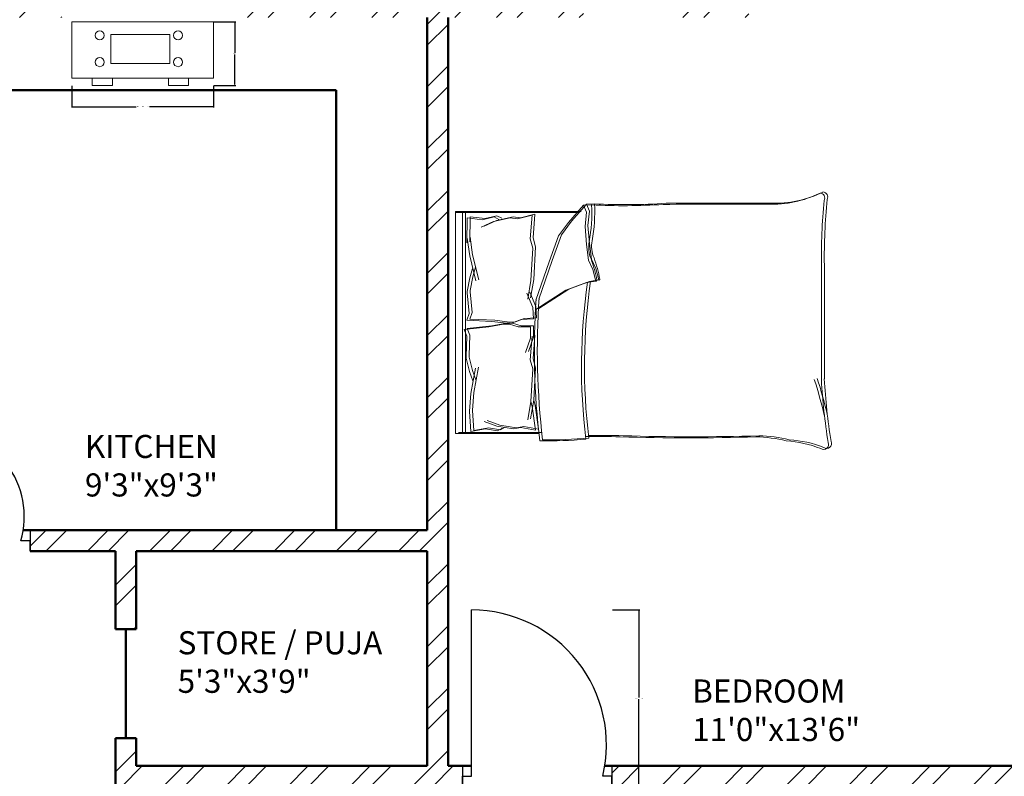
# Model space of a CAD drawing. Units: inches. Extents: x 963 to 2075, y 289 to 2657.
# Tile 96 of 98: x 1672 to 1885, y 2325 to 2489. Entities that reach past the tile are written whole.
import ezdxf

# ---------------------------------------------------------------- set-up
doc = ezdxf.new("R2010")
doc.units = ezdxf.units.IN
for name, color, linetype, lineweight in [('A-ANNO-DIMS', 2, 'Continuous', 18), ('A-AREA-IDEN', 7, 'Continuous', 18), ('A-DOOR', 4, 'Continuous', 25), ('A-FLOR-FIXT', 9, 'Continuous', 18), ('A-FURN', 8, 'Continuous', 18), ('A-WALL', 7, 'Continuous', 50), ('A-WALL-PATT', 8, 'Continuous', 13)]:
    doc.layers.add(name, color=color, linetype=linetype, lineweight=lineweight)
doc.styles.get("Standard").update_dxf_attribs({"font": 'arial.ttf'})
doc.dimstyles.get("Standard").update_dxf_attribs({"dimtxt": 0.18, "dimasz": 0.18, "dimexe": 0.18, "dimexo": 0.0625, "dimgap": 0.09, "dimtad": 0, "dimtih": 1, "dimtoh": 1, "dimdec": 4, "dimzin": 0, "dimdsep": 46, "dimtxsty": 'Standard', "dimcen": 0.09, "dimadec": 0, "dimazin": 0, "dimtfac": 1, "dimtdec": 4, "dimtofl": 0, "dimtmove": 0, "dimatfit": 3, "dimfxl": 1, "dimtolj": 1, "dimtzin": 0, "dimarcsym": 0})

# ---------------------------------------------------------------- blocks, each defined once
blk = doc.blocks.new('BED-DOUBLE')
for p, q in [((1236.12, 2450.52), (1254.23, 2450.52)), ((1236.12, 2450.52), (1254.23, 2450.52)), ((1236.76, 2450.75), (1254.87, 2450.75)), ((1236.76, 2450.75), (1254.87, 2450.75)), ((1238.25, 2444.94), (1237.53, 2450.04)), ((1237.53, 2450.04), (1240.71, 2449.46)), ((1238.25, 2444.94), (1237.53, 2450.04)), ((1237.53, 2450.04), (1240.71, 2449.46)), ((1245.77, 2450.18), (1244.76, 2449.61)), ((1245.77, 2450.18), (1244.76, 2449.61)), ((1248.37, 2449.75), (1245.77, 2450.18)), ((1248.37, 2449.75), (1245.77, 2450.18)), ((1250.92, 2450.1), (1247.74, 2449.52)), ((1250.92, 2450.1), (1247.74, 2449.52)), ((1251.56, 2450.33), (1248.37, 2449.75)), ((1251.56, 2450.33), (1248.37, 2449.75)), ((1250.89, 2450.1), (1251.22, 2445.82)), ((1250.89, 2450.1), (1251.22, 2445.82)), ((1251.53, 2450.32), (1251.86, 2446.04)), ((1251.53, 2450.32), (1251.86, 2446.04)), ((1252.7, 2450.52), (1252.7, 2402.73)), ((1252.7, 2450.52), (1252.7, 2402.73)), ((1253.34, 2450.75), (1253.34, 2402.96)), ((1253.34, 2450.75), (1253.34, 2402.96)), ((1254.87, 2450.75), (1254.87, 2402.73)), ((1237.61, 2444.71), (1236.89, 2449.81)), ((1236.89, 2449.81), (1240.07, 2449.23)), ((1237.61, 2444.71), (1236.89, 2449.81)), ((1236.89, 2449.81), (1240.07, 2449.23)), ((1240.07, 2449.23), (1241.66, 2449.52)), ((1240.07, 2449.23), (1241.66, 2449.52)), ((1240.71, 2449.46), (1242.3, 2449.75)), ((1240.71, 2449.46), (1242.3, 2449.75)), ((1241.66, 2449.52), (1245.28, 2448.94)), ((1241.66, 2449.52), (1245.28, 2448.94)), ((1242.3, 2449.75), (1245.92, 2449.17)), ((1242.3, 2449.75), (1245.92, 2449.17)), ((1245.13, 2449.96), (1244.12, 2449.38)), ((1245.13, 2449.96), (1244.12, 2449.38)), ((1247.74, 2449.52), (1245.13, 2449.96)), ((1247.74, 2449.52), (1245.13, 2449.96)), ((1245.28, 2448.94), (1248.02, 2447.93)), ((1245.28, 2448.94), (1248.02, 2447.93)), ((1245.92, 2449.17), (1248.66, 2448.16)), ((1245.92, 2449.17), (1248.66, 2448.16)), ((1238.6, 2447.61), (1237.94, 2443.58)), ((1238.6, 2447.61), (1237.94, 2443.58)), ((1239.24, 2447.84), (1238.58, 2443.81)), ((1239.24, 2447.84), (1238.58, 2443.81)), ((1251.22, 2445.82), (1251.21, 2445.71)), ((1251.22, 2445.82), (1251.21, 2445.71)), ((1251.84, 2445.94), (1251.56, 2442.11)), ((1251.84, 2445.94), (1251.56, 2442.11)), ((1251.86, 2446.04), (1251.84, 2445.94)), ((1251.86, 2446.04), (1251.84, 2445.94)), ((1237.94, 2443.58), (1237.61, 2444.71)), ((1237.94, 2443.58), (1237.61, 2444.71)), ((1238.58, 2443.81), (1238.15, 2436.8)), ((1238.58, 2443.81), (1238.15, 2436.8)), ((1238.58, 2443.81), (1238.25, 2444.94)), ((1238.58, 2443.81), (1238.25, 2444.94)), ((1251.21, 2445.71), (1250.92, 2441.89)), ((1251.21, 2445.71), (1250.92, 2441.89)), ((1237.94, 2443.58), (1237.51, 2436.57)), ((1237.94, 2443.58), (1237.51, 2436.57)), ((1250.92, 2441.89), (1249.9, 2436.39)), ((1250.92, 2441.89), (1249.9, 2436.39)), ((1251.56, 2442.11), (1250.54, 2436.62)), ((1251.56, 2442.11), (1250.54, 2436.62)), ((1251.12, 2439.37), (1251.84, 2437.34)), ((1251.12, 2439.37), (1251.84, 2437.34)), ((1174.99, 2438.93), (1174.99, 2414.32)), ((1174.99, 2438.93), (1174.99, 2414.32)), ((1175.63, 2439.16), (1175.63, 2414.55)), ((1175.63, 2439.16), (1175.63, 2414.55)), ((1250.48, 2439.14), (1251.21, 2437.12)), ((1250.48, 2439.14), (1251.21, 2437.12)), ((1251.84, 2437.34), (1252.57, 2434.45)), ((1251.84, 2437.34), (1252.57, 2434.45)), ((1237.51, 2436.57), (1238.06, 2434.61)), ((1237.51, 2436.57), (1238.06, 2434.61)), ((1238.15, 2436.8), (1238.7, 2434.84)), ((1238.15, 2436.8), (1238.7, 2434.84)), ((1251.21, 2437.12), (1251.93, 2434.22)), ((1251.21, 2437.12), (1251.93, 2434.23)), ((1238.06, 2434.61), (1237.66, 2429.48)), ((1238.06, 2434.61), (1237.66, 2429.48)), ((1237.97, 2429.89), (1239.06, 2433.04)), ((1237.97, 2429.89), (1239.06, 2433.04)), ((1238.7, 2434.84), (1238.3, 2429.71)), ((1238.7, 2434.84), (1238.3, 2429.71)), ((1238.61, 2430.12), (1239.7, 2433.26)), ((1238.61, 2430.12), (1239.7, 2433.26)), ((1251.93, 2433.9), (1251.78, 2429.46)), ((1251.93, 2433.9), (1251.78, 2429.46)), ((1251.93, 2434.23), (1251.93, 2433.9)), ((1251.93, 2434.22), (1251.93, 2433.9)), ((1252.57, 2434.13), (1252.42, 2429.69)), ((1252.57, 2434.13), (1252.42, 2429.69)), ((1252.57, 2434.45), (1252.57, 2434.13)), ((1252.57, 2434.45), (1252.57, 2434.13)), ((1237.97, 2427.43), (1237.97, 2429.89)), ((1237.97, 2427.43), (1237.97, 2429.89)), ((1238.61, 2427.66), (1238.61, 2430.12)), ((1238.61, 2427.66), (1238.61, 2430.12)), ((1251.78, 2429.46), (1252.36, 2428.01)), ((1251.78, 2429.46), (1252.36, 2428.01)), ((1252.42, 2429.69), (1253, 2428.24)), ((1252.42, 2429.69), (1253, 2428.24)), ((1240.65, 2427.43), (1237.97, 2427.43)), ((1240.65, 2427.43), (1237.97, 2427.43)), ((1241.29, 2427.66), (1238.61, 2427.66)), ((1241.29, 2427.66), (1238.61, 2427.66)), ((1242.53, 2426.86), (1240.65, 2427.43)), ((1242.53, 2426.86), (1240.65, 2427.43)), ((1242.49, 2426.79), (1240.66, 2426.09)), ((1242.49, 2426.79), (1240.66, 2426.09)), ((1243.17, 2427.08), (1241.29, 2427.66)), ((1243.17, 2427.08), (1241.29, 2427.66)), ((1243.15, 2426.64), (1241.86, 2426.56)), ((1243.15, 2426.64), (1241.86, 2426.56)), ((1243.79, 2426.87), (1242.49, 2426.79)), ((1243.79, 2426.87), (1242.49, 2426.79)), ((1243.83, 2426.86), (1242.53, 2426.86)), ((1243.83, 2426.86), (1242.53, 2426.86)), ((1246.37, 2426.26), (1243.15, 2426.64)), ((1246.37, 2426.26), (1243.15, 2426.64)), ((1244.47, 2427.08), (1243.17, 2427.08)), ((1244.47, 2427.08), (1243.17, 2427.08)), ((1247, 2426.49), (1243.79, 2426.87)), ((1247, 2426.49), (1243.79, 2426.87)), ((1247.01, 2427.43), (1243.83, 2426.86)), ((1247.01, 2427.43), (1243.83, 2426.86)), ((1247.65, 2427.66), (1244.47, 2427.08)), ((1247.65, 2427.66), (1244.47, 2427.08)), ((1252.36, 2428.01), (1247.01, 2427.43)), ((1252.36, 2428.01), (1247.01, 2427.43)), ((1253, 2428.24), (1247.65, 2427.66)), ((1253, 2428.24), (1247.65, 2427.66)), ((1240.02, 2425.86), (1237.34, 2425.7)), ((1240.02, 2425.86), (1237.34, 2425.7)), ((1237.34, 2425.7), (1237.49, 2423.24)), ((1237.34, 2425.7), (1237.49, 2423.24)), ((1240.66, 2426.09), (1237.98, 2425.93)), ((1240.66, 2426.09), (1237.98, 2425.93)), ((1237.98, 2425.93), (1238.13, 2423.47)), ((1237.98, 2425.93), (1238.13, 2423.47)), ((1241.86, 2426.56), (1240.02, 2425.86)), ((1241.86, 2426.56), (1240.02, 2425.86)), ((1251.74, 2426.02), (1246.37, 2426.26)), ((1251.74, 2426.02), (1246.37, 2426.26)), ((1252.38, 2426.25), (1247, 2426.49)), ((1252.38, 2426.25), (1247, 2426.49)), ((1251.25, 2424.54), (1251.74, 2426.02)), ((1251.25, 2424.54), (1251.74, 2426.02)), ((1251.68, 2420.11), (1251.25, 2424.54)), ((1251.68, 2420.11), (1251.25, 2424.54)), ((1251.89, 2424.77), (1252.38, 2426.25)), ((1251.89, 2424.77), (1252.38, 2426.25)), ((1252.31, 2420.34), (1251.89, 2424.77)), ((1252.31, 2420.34), (1251.89, 2424.77)), ((1236.85, 2423.74), (1230.36, 2419.55)), ((1236.85, 2423.74), (1230.36, 2419.55)), ((1237.49, 2423.96), (1231, 2419.77)), ((1237.49, 2423.96), (1231, 2419.77)), ((1237.49, 2423.24), (1238.78, 2420.17)), ((1237.49, 2423.24), (1238.78, 2420.17)), ((1238.13, 2423.47), (1239.42, 2420.4)), ((1238.13, 2423.47), (1239.42, 2420.4)), ((1233.92, 2413.35), (1236.85, 2421.69)), ((1233.92, 2413.35), (1236.85, 2421.69)), ((1234.56, 2413.58), (1237.49, 2421.92)), ((1234.56, 2413.58), (1237.49, 2421.92)), ((1238.6, 2421.43), (1237.94, 2417.4)), ((1238.6, 2421.43), (1237.94, 2417.4)), ((1239.24, 2421.66), (1238.58, 2417.63)), ((1239.24, 2421.66), (1238.58, 2417.63)), ((1252.33, 2420.02), (1252.31, 2420.34)), ((1252.33, 2420.02), (1252.31, 2420.34)), ((1226.51, 2418.07), (1224.49, 2417.76)), ((1226.51, 2418.07), (1224.49, 2417.76)), ((1230.36, 2419.55), (1225.87, 2417.84)), ((1230.36, 2419.55), (1225.87, 2417.84)), ((1231, 2419.77), (1226.51, 2418.07)), ((1231, 2419.77), (1226.51, 2418.07)), ((1251.15, 2416.86), (1251.7, 2419.79)), ((1251.15, 2416.86), (1251.7, 2419.79)), ((1251.7, 2419.79), (1251.68, 2420.11)), ((1251.7, 2419.79), (1251.68, 2420.11)), ((1251.79, 2417.09), (1252.33, 2420.02)), ((1251.79, 2417.09), (1252.33, 2420.02)), ((1225.87, 2417.84), (1223.86, 2417.53)), ((1225.87, 2417.84), (1223.86, 2417.53)), ((1223.86, 2417.53), (1224.47, 2415.05)), ((1223.86, 2417.53), (1224.47, 2415.05)), ((1224.49, 2417.76), (1225.11, 2415.28)), ((1224.49, 2417.76), (1225.11, 2415.28)), ((1237.94, 2417.4), (1237.51, 2410.39)), ((1237.94, 2417.4), (1237.51, 2410.39)), ((1238.58, 2417.63), (1238.15, 2410.62)), ((1238.58, 2417.63), (1238.15, 2410.62)), ((1251.16, 2412.08), (1249.81, 2417.5)), ((1251.16, 2412.08), (1249.81, 2417.5)), ((1251.8, 2412.31), (1250.45, 2417.73)), ((1251.8, 2412.31), (1250.45, 2417.73)), ((1250.56, 2414.79), (1251.15, 2416.86)), ((1250.56, 2414.79), (1251.15, 2416.86)), ((1251.2, 2415.02), (1251.79, 2417.09)), ((1251.2, 2415.02), (1251.79, 2417.09)), ((1224.47, 2415.05), (1225.4, 2413.04)), ((1224.47, 2415.05), (1225.4, 2413.04)), ((1225.11, 2415.28), (1226.04, 2413.27)), ((1225.11, 2415.28), (1226.04, 2413.27)), ((1225.4, 2413.04), (1225.87, 2409.63)), ((1225.4, 2413.04), (1225.87, 2409.63)), ((1226.04, 2413.27), (1226.51, 2409.86)), ((1226.04, 2413.27), (1226.51, 2409.86)), ((1231.9, 2407.77), (1233.92, 2413.35)), ((1231.9, 2407.78), (1233.92, 2413.35)), ((1232.54, 2408), (1234.56, 2413.58)), ((1232.54, 2408), (1234.56, 2413.58)), ((1251.69, 2408.28), (1251.16, 2412.08)), ((1251.69, 2408.28), (1251.16, 2412.08)), ((1252.33, 2408.51), (1251.8, 2412.31)), ((1252.33, 2408.51), (1251.8, 2412.31)), ((1225.87, 2409.63), (1226.18, 2405.76)), ((1225.87, 2409.63), (1226.18, 2405.76)), ((1226.51, 2409.86), (1226.82, 2405.99)), ((1226.51, 2409.86), (1226.82, 2405.99)), ((1237.51, 2410.39), (1238.06, 2408.43)), ((1237.51, 2410.39), (1238.06, 2408.43)), ((1238.15, 2410.62), (1238.7, 2408.66)), ((1238.15, 2410.62), (1238.7, 2408.66)), ((1252.31, 2404.11), (1252.41, 2409.51)), ((1252.31, 2404.11), (1252.41, 2409.51)), ((1252.41, 2409.51), (1252.33, 2408.51)), ((1252.41, 2409.51), (1252.33, 2408.51)), ((1229.74, 2404.83), (1231.9, 2407.78)), ((1229.74, 2404.83), (1231.9, 2407.77)), ((1230.38, 2405.06), (1232.54, 2408)), ((1230.38, 2405.06), (1232.54, 2408)), ((1238.06, 2408.43), (1237.66, 2403.3)), ((1238.06, 2408.43), (1237.66, 2403.3)), ((1238.7, 2408.66), (1238.3, 2403.52)), ((1238.7, 2408.66), (1238.3, 2403.52)), ((1251.68, 2403.88), (1251.77, 2409.29)), ((1251.68, 2403.88), (1251.77, 2409.28)), ((1251.77, 2409.29), (1251.69, 2408.28)), ((1251.77, 2409.28), (1251.69, 2408.28)), ((1226.18, 2405.76), (1225.87, 2402.66)), ((1226.18, 2405.76), (1225.87, 2402.66)), ((1226.82, 2405.99), (1226.51, 2402.89)), ((1226.82, 2405.99), (1226.51, 2402.89)), ((1245.98, 2404.69), (1248.65, 2405.87)), ((1245.98, 2404.69), (1248.65, 2405.87)), ((1246.61, 2404.91), (1249.29, 2406.1)), ((1246.61, 2404.91), (1249.29, 2406.09)), ((1226.49, 2401.13), (1229.74, 2404.83)), ((1226.49, 2401.13), (1229.74, 2404.83)), ((1227.13, 2401.36), (1230.38, 2405.06)), ((1227.13, 2401.36), (1230.38, 2405.06)), ((1237.66, 2403.3), (1240.8, 2404.07)), ((1237.66, 2403.3), (1240.8, 2404.07)), ((1238.3, 2403.52), (1241.44, 2404.3)), ((1238.3, 2403.52), (1241.44, 2404.3)), ((1240.8, 2404.07), (1242.4, 2403.88)), ((1240.8, 2404.07), (1242.4, 2403.88)), ((1241.44, 2404.3), (1243.04, 2404.11)), ((1241.44, 2404.3), (1243.04, 2404.11)), ((1242.4, 2403.88), (1245.98, 2404.69)), ((1242.4, 2403.88), (1245.98, 2404.69)), ((1243.04, 2404.11), (1246.61, 2404.91)), ((1243.04, 2404.11), (1246.61, 2404.91)), ((1245.89, 2403.67), (1244.85, 2404.18)), ((1245.89, 2403.67), (1244.85, 2404.18)), ((1246.53, 2403.89), (1245.49, 2404.41)), ((1246.53, 2403.89), (1245.49, 2404.41)), ((1248.46, 2404.26), (1245.89, 2403.67)), ((1248.46, 2404.26), (1245.89, 2403.67)), ((1249.1, 2404.49), (1246.53, 2403.89)), ((1249.1, 2404.49), (1246.53, 2403.89)), ((1251.68, 2403.88), (1248.46, 2404.26)), ((1251.68, 2403.88), (1248.46, 2404.26)), ((1252.31, 2404.11), (1249.1, 2404.49)), ((1252.31, 2404.11), (1249.1, 2404.49)), ((1224.74, 2401.05), (1226.49, 2401.13, 3.87)), ((1224.74, 2401.05), (1226.49, 2401.13, 3.87)), ((1225.38, 2401.28), (1227.13, 2401.36, 3.87)), ((1225.38, 2401.28), (1227.13, 2401.36, 3.87)), ((1225.87, 2402.66), (1226.49, 2401.13)), ((1225.87, 2402.66), (1226.49, 2401.13)), ((1226.51, 2402.89), (1227.13, 2401.36)), ((1226.51, 2402.89), (1227.13, 2401.36)), ((1254.23, 2402.73), (1227.62, 2402.73)), ((1254.23, 2402.73), (1227.62, 2402.73)), ((1254.87, 2402.96), (1228.26, 2402.96)), ((1254.87, 2402.96), (1228.26, 2402.96)), ((1254.87, 2402.73), (1254.23, 2402.73))]:
    blk.add_line(p, q)
for centre, radius, start, end in [((1174.51, 2452.91), 1.09, 56.1736, 203.4781), ((1174.51, 2452.91), 1.09, 56.1736, 203.4781), ((1053.4, 2432.57), 121.76, 2.9958, 9.4091), ((1053.4, 2432.57), 121.76, 2.9958, 9.4091), ((1175.15, 2453.14), 1.09, 56.1736, 203.4781), ((1175.15, 2453.14), 1.09, 56.1736, 203.4781), ((1054.03, 2432.8), 121.76, 2.9958, 9.4091), ((1054.03, 2432.8), 121.76, 2.9958, 9.4091), ((1183.96, 2475.65), 23.56, 247.9751, 266.652), ((1183.96, 2475.65), 23.56, 247.9751, 266.652), ((1184.6, 2475.88), 23.56, 247.9751, 266.652), ((1184.6, 2475.88), 23.56, 247.9751, 266.652), ((1190.36, 2481.12), 29.63, 256.0648, 268.9113), ((1190.36, 2481.12), 29.63, 256.0648, 268.9113), ((1234.78, 2369.06), 83.31, 88.7218, 95.604), ((1234.78, 2369.06), 83.31, 88.7218, 95.604), ((1072.82, 2432.86), 164.97, 356.0865, 6.7821), ((1072.82, 2432.86), 164.97, 356.0865, 6.7821), ((1189.72, 2480.89), 29.63, 256.0648, 268.9113), ((1189.72, 2480.89), 29.63, 256.0648, 268.9113), ((1203.62, 1969.17), 482.31, 88.2277, 91.7185), ((1203.62, 1969.17), 482.31, 88.2277, 91.7185), ((1204.26, 1969.4), 482.31, 88.2277, 91.7185), ((1204.26, 1969.4), 482.31, 88.2277, 91.7185), ((1223.06, 2621.3), 170.11, 268.4762, 271.0082), ((1223.06, 2621.3), 170.11, 268.4762, 271.0082), ((1223.7, 2621.53), 170.11, 268.4762, 271.0082), ((1223.7, 2621.53), 170.11, 268.4762, 271.0082), ((1097.92, 2436.24), 129.02, 351.7845, 6.9006), ((1097.92, 2436.24), 129.02, 351.7845, 6.9006), ((1234.14, 2368.83), 83.31, 88.7218, 95.604), ((1234.14, 2368.83), 83.31, 88.7218, 95.604), ((1098.56, 2436.47), 129.02, 351.7845, 6.9006), ((1098.56, 2436.47), 129.02, 351.7845, 6.9006), ((1072.18, 2432.64), 164.97, 356.0865, 6.7821), ((1072.18, 2432.64), 164.97, 356.0865, 6.7821), ((1277.94, 2471.22), 106.46, 193.3832, 197.7053), ((1277.94, 2471.22), 106.46, 193.3832, 197.7053), ((1278.58, 2471.44), 106.46, 193.3832, 197.7053), ((1278.58, 2471.44), 106.46, 193.3832, 197.7053), ((1223.79, 2417.36), 0.185, 70.2464, 181.1377), ((1223.79, 2417.36), 0.185, 70.2464, 181.1377), ((1252.75, 2422.84), 29.65, 190.6617, 199.8806), ((1252.75, 2422.84), 29.65, 190.6617, 199.8806), ((1224.43, 2417.59), 0.185, 70.2464, 181.1377), ((1224.43, 2417.59), 0.185, 70.2464, 181.1377), ((1253.39, 2423.07), 29.65, 190.6617, 199.8806), ((1253.39, 2423.07), 29.65, 190.6617, 199.8806), ((1041.96, 2412.84), 133.04, 354.4998, 0.6351), ((1041.96, 2412.84), 133.04, 354.4998, 0.6351), ((1042.6, 2413.07), 133.04, 354.4998, 0.6351), ((1042.6, 2413.07), 133.04, 354.4998, 0.6351), ((1219.17, 2410.25), 6.22, 348.6608, 23.7384), ((1219.17, 2410.25), 6.22, 348.6608, 23.7384), ((1219.81, 2410.48), 6.22, 348.6608, 23.7384), ((1219.81, 2410.48), 6.22, 348.6608, 23.7384), ((1260.89, 2402.67), 36.18, 169.8763, 182.5657), ((1260.89, 2402.67), 36.18, 169.8763, 182.5657), ((1261.53, 2402.9), 36.18, 169.8763, 182.5657), ((1261.53, 2402.9), 36.18, 169.8763, 182.5657), ((1186.21, 2378.07), 23.07, 87.4714, 116.4681), ((1186.21, 2378.07), 23.07, 87.4714, 116.4681), ((1187.05, 6962.97), 4561.86, 270.00217, 270.28689), ((1187.05, 6962.97), 4561.86, 270.00217, 270.28689), ((1217.92, 2271.73), 129.5, 86.9791, 93.8365), ((1217.92, 2271.73), 129.5, 86.9791, 93.8365), ((1218.56, 2271.96), 129.5, 86.9791, 93.8365), ((1218.56, 2271.96), 129.5, 86.9791, 93.8365), ((1175.36, 2399.58), 1.1, 152.6588, 266.02), ((1175.36, 2399.58), 1.1, 152.6588, 266.02), ((1176, 2399.81), 1.1, 152.6588, 266.02), ((1176, 2399.81), 1.1, 152.6588, 266.02), ((1185.57, 2377.84), 23.07, 87.4714, 116.4681), ((1185.57, 2377.84), 23.07, 87.4714, 116.4681), ((1186.41, 6962.74), 4561.86, 270.00217, 270.28689), ((1186.41, 6962.74), 4561.86, 270.00217, 270.28689)]:
    blk.add_arc(centre, radius, start, end)
blk = doc.blocks.new('KITCHEN-SINK')
for points in [[(-0.1, 14), (30.59, 14), (30.59, 1.84), (-0.1, 1.84)], [(8.33, 11.28), (21.1, 11.28), (21.1, 5.02), (8.33, 5.02)], [(4.31, 1.84), (8.69, 1.84), (8.69, 0.24), (4.31, 0.24)], [(20.79, 1.84), (25.17, 1.84), (25.17, 0.24), (20.79, 0.24)]]:
    blk.add_lwpolyline(points, close=True)
for centre in [(5.94, 11.08), (22.9, 11.08), (5.94, 5.28), (22.9, 5.28)]:
    blk.add_circle(centre, 0.978)
blk = doc.blocks.new('DOOR-3')
for p, q in [((2, 2.25), (2, 38.25)), ((0, 4.5), (0, 0)), ((32.39, 4.5), (32.39, 0)), ((0, 0), (0, 2.25)), ((0, 2.25), (2, 2.25)), ((32.39, 2.25), (30.39, 2.25)), ((32.39, 0), (32.39, 2.25))]:
    blk.add_line(p, q)
blk.add_arc((2, 9.06), 29.19, 346.5105, 90)
blk = doc.blocks.new('*D20')
at = {"layer": 'A-ANNO-DIMS', "color": 0, "lineweight": -2, "transparency": 16777216}
for p, q in [((1683.48, 2474.56), (1683.48, 2469.84)), ((1714.16, 2474.56), (1714.16, 2469.84)), ((1683.66, 2470.02), (1697.38, 2470.02)), ((1713.98, 2470.02), (1700.26, 2470.02))]:
    blk.add_line(p, q, dxfattribs=at)
at = {"layer": 'A-ANNO-DIMS', "color": 0, "transparency": 16777216}
for points in [[(1683.66, 2470.05), (1683.66, 2469.99), (1683.48, 2470.02)], [(1713.98, 2470.05), (1713.98, 2469.99), (1714.16, 2470.02)]]:
    blk.add_solid(points, dxfattribs=at)
at = {"layer": 'Defpoints', "color": 0, "transparency": 16777216}
for p in [(1683.48, 2474.62), (1714.16, 2474.62), (1714.16, 2470.02)]:
    blk.add_point(p, dxfattribs=at)
at = {"layer": 'A-ANNO-DIMS', "color": 0, "transparency": 16777216, "insert": (1698.82, 2470.02), "char_height": 0.18, "attachment_point": 5}
blk.add_mtext('\\A1;KITCHEN SINK 31 TYP.', dxfattribs=at)
blk = doc.blocks.new('*D21')
at = {"layer": 'A-ANNO-DIMS', "color": 0, "lineweight": -2, "transparency": 16777216}
for p, q in [((1714.23, 2488.38), (1718.95, 2488.38)), ((1718.77, 2488.2), (1718.77, 2481.68)), ((1718.77, 2474.8), (1718.77, 2481.32)), ((1714.23, 2474.62), (1718.95, 2474.62))]:
    blk.add_line(p, q, dxfattribs=at)
at = {"layer": 'A-ANNO-DIMS', "color": 0, "transparency": 16777216}
for points in [[(1718.74, 2488.2), (1718.8, 2488.2), (1718.77, 2488.38)], [(1718.74, 2474.8), (1718.8, 2474.8), (1718.77, 2474.62)]]:
    blk.add_solid(points, dxfattribs=at)
at = {"layer": 'Defpoints', "color": 0, "transparency": 16777216}
for p in [(1714.16, 2488.38), (1718.77, 2488.38), (1714.16, 2474.62)]:
    blk.add_point(p, dxfattribs=at)
at = {"layer": 'A-ANNO-DIMS', "color": 0, "transparency": 16777216, "insert": (1718.77, 2481.5), "char_height": 0.18, "attachment_point": 5}
blk.add_mtext('\\A1;14 TYP.', dxfattribs=at)
blk = doc.blocks.new('*D34')
at = {"layer": 'A-ANNO-DIMS', "color": 0, "lineweight": -2, "transparency": 16777216}
for p, q in [((1800.57, 2361.07), (1806.43, 2361.07)), ((1806.25, 2360.89), (1806.25, 2342.13)), ((1806.25, 2323), (1806.25, 2341.76)), ((1800.57, 2322.82), (1806.43, 2322.82))]:
    blk.add_line(p, q, dxfattribs=at)
at = {"layer": 'A-ANNO-DIMS', "color": 0, "transparency": 16777216}
for points in [[(1806.22, 2360.89), (1806.28, 2360.89), (1806.25, 2361.07)], [(1806.22, 2323), (1806.28, 2323), (1806.25, 2322.82)]]:
    blk.add_solid(points, dxfattribs=at)
at = {"layer": 'Defpoints', "color": 0, "transparency": 16777216}
for p in [(1800.51, 2361.07), (1806.25, 2361.07), (1800.51, 2322.82)]:
    blk.add_point(p, dxfattribs=at)
at = {"layer": 'A-ANNO-DIMS', "color": 0, "transparency": 16777216, "insert": (1806.25, 2341.94), "char_height": 0.18, "attachment_point": 5}
blk.add_mtext('\\A1;DOOR D3 38 TYP.', dxfattribs=at)

msp = doc.modelspace()

# ---------------------------------------------------------------- hatches: boundary and pattern name
at = {"layer": 'A-WALL-PATT'}
h = msp.add_hatch(dxfattribs=at)
h.set_pattern_fill('ANSI32', color=256)
h.paths.add_polyline_path([(1296.92, 2558.32), (1203.92, 2558.32), (1203.92, 2493.82), (1191.53, 2493.82), (1191.53, 2489.32), (1211.06, 2489.32), (1211.06, 2492.02), (1211.06, 2493.82), (1208.42, 2493.82), (1208.42, 2553.82), (1292.42, 2553.82), (1292.42, 2538.86), (1296.92, 2538.86)])
h.paths.add_polyline_path([(1442.42, 2558.32), (1349.42, 2558.32), (1349.42, 2538.94), (1353.92, 2538.94), (1353.92, 2553.82), (1437.92, 2553.82), (1437.92, 2493.82), (1434.54, 2493.82), (1434.54, 2489.32), (1448.31, 2489.32), (1448.31, 2491.57), (1448.31, 2493.82), (1442.42, 2493.82)])
h.paths.add_polyline_path([(1415.55, 2491.57), (1415.55, 2493.82), (1340.94, 2493.82), (1340.94, 2489.32), (1371.92, 2489.32), (1371.92, 2378.32), (1367.6, 2378.32), (1367.6, 2373.82), (1371.92, 2373.82), (1371.92, 2355.19), (1376.42, 2355.19), (1376.42, 2489.32), (1415.55, 2489.32)])
h.paths.add_polyline_path([(1304.94, 2491.57), (1304.94, 2493.82), (1296.92, 2493.82), (1296.92, 2514.86), (1292.42, 2514.86), (1292.42, 2493.82), (1232.81, 2493.82), (1232.81, 2489.32), (1256.42, 2489.32), (1256.42, 2327.32), (1253.71, 2327.32), (1253.71, 2322.82), (1328.42, 2322.82), (1328.42, 2331.15), (1323.92, 2331.15), (1323.92, 2327.32), (1260.92, 2327.32), (1260.92, 2373.82), (1323.92, 2373.82), (1323.92, 2357.81), (1328.42, 2357.81), (1328.42, 2373.82), (1346.01, 2373.82), (1346.01, 2376.07), (1346.01, 2378.32), (1260.92, 2378.32), (1260.92, 2489.32), (1304.94, 2489.32)])
h.paths.add_polyline_path([(1226.65, 2327.32), (1124.42, 2327.32), (1124.42, 2347.45), (1119.92, 2347.45), (1119.92, 2322.82), (1163.42, 2322.82), (1163.42, 2305.43), (1165.67, 2305.43), (1167.92, 2305.43), (1167.92, 2322.82), (1226.65, 2322.82), (1226.65, 2325.07)])
h.paths.add_polyline_path([(1095.92, 2489.32), (1124.42, 2489.32), (1131.53, 2489.32), (1131.53, 2491.57), (1131.53, 2493.82), (1119.92, 2493.82), (1091.42, 2493.82), (1091.42, 2417.32), (1095.92, 2417.32), (1119.92, 2417.32), (1119.92, 2407.45), (1124.42, 2407.45), (1124.42, 2421.82), (1095.92, 2421.82)])
h.paths.add_polyline_path([(1512.92, 2558.32), (1508.42, 2558.32), (1508.42, 2493.82), (1503.4, 2493.82), (1503.4, 2489.32), (1508.42, 2489.32), (1508.42, 2327.32), (1376.42, 2327.32), (1376.42, 2330.27), (1371.92, 2330.27), (1371.92, 2298.74), (1376.42, 2298.74), (1376.42, 2322.82), (1508.42, 2322.82), (1508.42, 2165.32), (1504.26, 2165.32), (1504.26, 2160.82), (1508.42, 2160.82), (1508.42, 2108.32), (1512.92, 2108.32), (1512.92, 2160.82), (1516.18, 2160.82), (1516.18, 2163.07), (1516.18, 2165.32), (1512.92, 2165.32), (1512.92, 2322.82), (1644.92, 2322.82), (1644.92, 2298.74), (1649.42, 2298.74), (1649.42, 2322.82), (1649.42, 2330.94), (1647.17, 2330.94), (1644.92, 2330.94), (1644.92, 2327.32), (1512.92, 2327.32), (1512.92, 2489.32), (1516.76, 2489.32), (1516.76, 2491.57), (1516.76, 2493.82), (1512.92, 2493.82)])
h.paths.add_polyline_path([(1671.92, 2558.32), (1578.92, 2558.32), (1578.92, 2493.82), (1573.53, 2493.82), (1573.53, 2489.32), (1586.54, 2489.32), (1586.54, 2491.57), (1586.54, 2493.82), (1583.42, 2493.82), (1583.42, 2553.82), (1667.42, 2553.82), (1667.42, 2541.11), (1671.92, 2541.11)])
h.paths.add_polyline_path([(1681.26, 2493.82), (1671.92, 2493.82), (1671.92, 2517.11), (1667.42, 2517.11), (1667.42, 2493.82), (1610.22, 2493.82), (1610.22, 2489.32), (1644.92, 2489.32), (1644.92, 2357.87), (1649.42, 2357.87), (1649.42, 2373.82), (1652.2, 2373.82), (1652.2, 2375.83), (1652.2, 2378.32), (1649.42, 2378.32), (1649.42, 2489.32), (1681.26, 2489.32), (1681.26, 2491.57)])
h.paths.add_polyline_path([(1821.92, 2558.32), (1728.92, 2558.32), (1728.92, 2541), (1733.42, 2541), (1733.42, 2553.82), (1817.42, 2553.82), (1817.42, 2493.82), (1813.51, 2493.82), (1813.51, 2489.32), (1830.08, 2489.32), (1830.08, 2491.57), (1830.08, 2493.82), (1821.92, 2493.82)])
h.paths.add_polyline_path([(1794.24, 2493.82), (1717.26, 2493.82), (1717.26, 2489.32), (1760.42, 2489.32), (1760.42, 2378.32), (1674.4, 2378.32), (1674.4, 2373.82), (1692.92, 2373.82), (1692.92, 2356.95), (1697.42, 2356.95), (1697.42, 2373.82), (1760.42, 2373.82), (1760.42, 2327.32), (1697.42, 2327.32), (1697.42, 2333.34), (1692.92, 2333.34), (1692.92, 2322.82), (1768.04, 2322.82), (1768.04, 2325.07), (1768.04, 2327.32), (1764.92, 2327.32), (1764.92, 2489.32), (1794.24, 2489.32)])
h.paths.add_polyline_path([(1733.42, 2517), (1728.92, 2517), (1728.92, 2493.82), (1733.42, 2493.82)], flags=17)
h.paths.add_polyline_path([(1929.92, 2493.82), (1890.08, 2493.82), (1890.08, 2489.32), (1896.92, 2489.32), (1925.42, 2489.32), (1925.42, 2421.82), (1896.92, 2421.82), (1896.92, 2408.32), (1901.42, 2408.32), (1901.42, 2417.32), (1925.42, 2417.32), (1929.92, 2417.32)])
h.paths.add_polyline_path([(1901.42, 2348.32), (1896.92, 2348.32), (1896.92, 2327.32), (1800.42, 2327.32), (1800.42, 2322.82), (1853.42, 2322.82), (1853.42, 2309.45), (1857.92, 2309.45), (1857.92, 2322.82), (1901.42, 2322.82)])
h.paths.add_polyline_path([(1857.92, 2249.45), (1853.42, 2249.45), (1853.42, 2214.82), (1686.31, 2214.82), (1686.31, 2210.32), (1853.42, 2210.32), (1853.42, 2202.13), (1857.92, 2202.13), (1857.92, 2210.32)])
h.paths.add_polyline_path([(1857.92, 2142.13), (1853.42, 2142.13), (1853.42, 2115.42), (1841.42, 2115.42), (1841.42, 2088.53), (1841.42, 2046.95), (1845.92, 2046.95), (1845.92, 2110.92), (1905.92, 2110.92), (1905.92, 2092.52), (1910.42, 2092.52), (1910.42, 2115.42), (1857.92, 2115.42)])
h.paths.add_polyline_path([(1532.44, 1482.34), (1573.46, 1482.34), (1573.46, 1501), (1532.44, 1501)], flags=9)
h.paths.add_polyline_path([(1438.66, 1486.3), (1479.68, 1486.3), (1479.68, 1504.96), (1438.66, 1504.96)], flags=9)
h.paths.add_polyline_path([(1411.22, 1365.31), (1659.14, 1365.31), (1659.14, 1402.4), (1411.22, 1402.4)], flags=9)
h.paths.add_polyline_path([(1185.67, 2296.3), (1248.16, 2296.3), (1248.16, 2314.95), (1185.67, 2314.95)], flags=9)
h.paths.add_polyline_path([(1177.31, 2187.35), (1216.15, 2187.35), (1216.15, 2206.01), (1177.31, 2206.01)], flags=9)
h.paths.add_polyline_path([(1295.1, 1602.08), (1328.26, 1602.08), (1328.26, 1620.74), (1295.1, 1620.74)], flags=9)
h.paths.add_polyline_path([(1525.13, 2005.99), (1558.39, 2005.99), (1558.39, 2024.65), (1525.13, 2024.65)], flags=9)
h.paths.add_polyline_path([(1459.61, 1977.13), (1472.19, 1977.13), (1472.19, 1987.43), (1459.61, 1987.43)], flags=9)
h.paths.add_polyline_path([(1467.81, 2053.68), (1480.02, 2053.68), (1480.02, 2063.98), (1467.81, 2063.98)], flags=9)
h.paths.add_polyline_path([(1555.18, 2119.02), (1584.56, 2119.02), (1584.56, 2137.68), (1555.18, 2137.68)], flags=25)
h.paths.add_polyline_path([(1405.39, 2115.29), (1444.48, 2115.29), (1444.48, 2133.95), (1405.39, 2133.95)], flags=25)
h.paths.add_polyline_path([(1698.48, 2004.26), (1727.69, 2004.26), (1727.69, 2022.92), (1698.48, 2022.92)], flags=9)
h.paths.add_polyline_path([(1612.16, 1972.86), (1629.02, 1972.86), (1629.02, 1983.16), (1612.16, 1983.16)], flags=9)
h.paths.add_polyline_path([(1608.29, 2060.04), (1625.15, 2060.04), (1625.15, 2070.34), (1608.29, 2070.34)], flags=9)
h.paths.add_polyline_path([(1527.95, 1684.4), (1566.79, 1684.4), (1566.79, 1703.06), (1527.95, 1703.06)], flags=9)
h.paths.add_polyline_path([(1422.79, 1683.59), (1461.63, 1683.59), (1461.63, 1702.25), (1422.79, 1702.25)], flags=9)
h.paths.add_polyline_path([(1531.26, 1732.46), (1574.01, 1732.46), (1574.01, 1751.12), (1531.26, 1751.12)], flags=9)
h.paths.add_polyline_path([(1402.87, 1732.85), (1439.8, 1732.85), (1439.8, 1751.5), (1402.87, 1751.5)], flags=9)
h.paths.add_polyline_path([(1243.12, 1923.13), (1281.96, 1923.13), (1281.96, 1941.79), (1243.12, 1941.79)], flags=9)
h.paths.add_polyline_path([(1181.75, 1792.27), (1244.24, 1792.27), (1244.24, 1810.93), (1181.75, 1810.93)], flags=9)
h.paths.add_polyline_path([(1265.82, 1670.3), (1316.07, 1670.3), (1316.07, 1688.96), (1265.82, 1688.96)], flags=9)
h.paths.add_polyline_path([(1140.26, 1676.05), (1179.1, 1676.05), (1179.1, 1694.71), (1140.26, 1694.71)], flags=9)
h.paths.add_polyline_path([(1107.49, 1490.89), (1143.37, 1490.89), (1143.37, 1509.55), (1107.49, 1509.55)], flags=9)
h.paths.add_polyline_path([(1217.58, 1483.9), (1246.74, 1483.9), (1246.74, 1502.56), (1217.58, 1502.56)], flags=9)
h.paths.add_polyline_path([(1389.21, 1486.92), (1418.37, 1486.92), (1418.37, 1505.58), (1389.21, 1505.58)], flags=9)
h.paths.add_polyline_path([(1672.21, 1602.08), (1705.37, 1602.08), (1705.37, 1620.74), (1672.21, 1620.74)], flags=9)
h.paths.add_polyline_path([(1752.08, 1522.64), (1781.24, 1522.64), (1781.24, 1541.3), (1752.08, 1541.3)], flags=9)
h.paths.add_polyline_path([(1848.27, 1491.26), (1884.16, 1491.26), (1884.16, 1509.92), (1848.27, 1509.92)], flags=9)
h.paths.add_polyline_path([(1822.47, 1685.62), (1861.31, 1685.62), (1861.31, 1704.28), (1822.47, 1704.28)], flags=9)
h.paths.add_polyline_path([(1713.19, 1672.23), (1763.44, 1672.23), (1763.44, 1690.89), (1713.19, 1690.89)], flags=9)
h.paths.add_polyline_path([(1736.62, 1790.58), (1799.11, 1790.58), (1799.11, 1809.24), (1736.62, 1809.24)], flags=9)
h.paths.add_polyline_path([(1691.49, 1916.36), (1730.33, 1916.36), (1730.33, 1935.01), (1691.49, 1935.01)], flags=9)
h.paths.add_polyline_path([(1764.87, 1973.92), (1794.31, 1973.92), (1794.31, 1992.58), (1764.87, 1992.58)], flags=9)
h.paths.add_polyline_path([(1767.85, 2034.02), (1797.29, 2034.02), (1797.29, 2052.67), (1767.85, 2052.67)], flags=9)
h.paths.add_polyline_path([(1851.59, 2060.33), (1880.75, 2060.33), (1880.75, 2078.99), (1851.59, 2078.99)], flags=25)
h.paths.add_polyline_path([(1688.49, 2086.87), (1727.33, 2086.87), (1727.33, 2105.53), (1688.49, 2105.53)], flags=9)
h.paths.add_polyline_path([(1537.74, 2293.58), (1580.49, 2293.58), (1580.49, 2312.24), (1537.74, 2312.24)], flags=25)
h.paths.add_polyline_path([(1425.59, 2296.11), (1468.34, 2296.11), (1468.34, 2314.77), (1425.59, 2314.77)], flags=25)
h.paths.add_polyline_path([(1278.52, 2004.18), (1307.72, 2004.18), (1307.72, 2022.84), (1278.52, 2022.84)], flags=9)
h.paths.add_polyline_path([(1193.28, 1973.63), (1222.72, 1973.63), (1222.72, 1992.29), (1193.28, 1992.29)], flags=9)
h.paths.add_polyline_path([(1192.41, 2040.58), (1221.84, 2040.58), (1221.84, 2059.23), (1192.41, 2059.23)], flags=9)
h.paths.add_polyline_path([(1130.6, 1951.39), (1159.76, 1951.39), (1159.76, 1970.05), (1130.6, 1970.05)], flags=9)
h.paths.add_polyline_path([(1132.83, 2052.49), (1161.98, 2052.49), (1161.98, 2071.15), (1132.83, 2071.15)], flags=9)
h.paths.add_polyline_path([(1265.13, 2334.62), (1315.38, 2334.62), (1315.38, 2353.28), (1265.13, 2353.28)], flags=25)
h.paths.add_polyline_path([(1136.74, 2330.79), (1175.58, 2330.79), (1175.58, 2349.44), (1136.74, 2349.44)], flags=9)
h.paths.add_polyline_path([(1287.42, 2417.2), (1320.58, 2417.2), (1320.58, 2435.86), (1287.42, 2435.86)], flags=25)
h.paths.add_polyline_path([(1430.99, 2329.16), (1469.83, 2329.16), (1469.83, 2347.82), (1430.99, 2347.82)], flags=25)
h.paths.add_polyline_path([(1525.42, 2329.21), (1564.26, 2329.21), (1564.26, 2347.87), (1525.42, 2347.87)], flags=25)
h.paths.add_polyline_path([(1684.52, 2382.8), (1717.68, 2382.8), (1717.68, 2401.46), (1684.52, 2401.46)], flags=25)
h.paths.add_polyline_path([(1704.81, 2340.29), (1755.05, 2340.29), (1755.05, 2358.95), (1704.81, 2358.95)], flags=25)
h.paths.add_polyline_path([(1694.11, 2287.76), (1756.6, 2287.76), (1756.6, 2306.41), (1694.11, 2306.41)], flags=9)
h.paths.add_polyline_path([(1815.78, 2329.86), (1854.62, 2329.86), (1854.62, 2348.52), (1815.78, 2348.52)], flags=9)
h.paths.add_polyline_path([(1842.87, 2514.26), (1878.76, 2514.26), (1878.76, 2532.91), (1842.87, 2532.91)], flags=9)
h.paths.add_polyline_path([(1769.51, 2531.45), (1798.67, 2531.45), (1798.67, 2550.1), (1769.51, 2550.1)], flags=25)
h.paths.add_polyline_path([(1594.77, 2518.47), (1623.93, 2518.47), (1623.93, 2537.13), (1594.77, 2537.13)], flags=25)
h.paths.add_polyline_path([(1520.72, 2516.18), (1556.61, 2516.18), (1556.61, 2534.84), (1520.72, 2534.84)], flags=25)
h.paths.add_polyline_path([(1464.46, 2516.69), (1500.34, 2516.69), (1500.34, 2535.35), (1464.46, 2535.35)], flags=25)
h.paths.add_polyline_path([(1365.7, 2528.97), (1394.85, 2528.97), (1394.85, 2547.63), (1365.7, 2547.63)], flags=25)
h.paths.add_polyline_path([(1222.84, 2516.23), (1252, 2516.23), (1252, 2534.89), (1222.84, 2534.89)], flags=25)
h.paths.add_polyline_path([(1104.55, 2509.6), (1140.43, 2509.6), (1140.43, 2528.26), (1104.55, 2528.26)], flags=9)
h = msp.add_hatch(dxfattribs=at)
h.set_pattern_fill('ANSI32', color=256)
h.paths.add_polyline_path([(1335.97, 2212.57), (1335.97, 2214.82), (1167.92, 2214.82), (1167.92, 2245.43), (1163.42, 2245.43), (1163.42, 2210.32), (1163.42, 2194.81), (1167.92, 2194.81), (1167.92, 2210.32), (1335.97, 2210.32)])
h.paths.add_polyline_path([(1532.44, 1482.34), (1573.46, 1482.34), (1573.46, 1501), (1532.44, 1501)], flags=9)
h.paths.add_polyline_path([(1438.66, 1486.3), (1479.68, 1486.3), (1479.68, 1504.96), (1438.66, 1504.96)], flags=9)
h.paths.add_polyline_path([(1411.22, 1365.31), (1659.14, 1365.31), (1659.14, 1402.4), (1411.22, 1402.4)], flags=9)
h.paths.add_polyline_path([(1185.67, 2296.3), (1248.16, 2296.3), (1248.16, 2314.95), (1185.67, 2314.95)], flags=9)
h.paths.add_polyline_path([(1177.31, 2187.35), (1216.15, 2187.35), (1216.15, 2206.01), (1177.31, 2206.01)], flags=9)
h.paths.add_polyline_path([(1295.1, 1602.08), (1328.26, 1602.08), (1328.26, 1620.74), (1295.1, 1620.74)], flags=9)
h.paths.add_polyline_path([(1525.13, 2005.99), (1558.39, 2005.99), (1558.39, 2024.65), (1525.13, 2024.65)], flags=9)
h.paths.add_polyline_path([(1459.61, 1977.13), (1472.19, 1977.13), (1472.19, 1987.43), (1459.61, 1987.43)], flags=9)
h.paths.add_polyline_path([(1467.81, 2053.68), (1480.02, 2053.68), (1480.02, 2063.98), (1467.81, 2063.98)], flags=9)
h.paths.add_polyline_path([(1555.18, 2119.02), (1584.56, 2119.02), (1584.56, 2137.68), (1555.18, 2137.68)], flags=9)
h.paths.add_polyline_path([(1405.39, 2115.29), (1444.48, 2115.29), (1444.48, 2133.95), (1405.39, 2133.95)], flags=9)
h.paths.add_polyline_path([(1698.48, 2004.26), (1727.69, 2004.26), (1727.69, 2022.92), (1698.48, 2022.92)], flags=9)
h.paths.add_polyline_path([(1612.16, 1972.86), (1629.02, 1972.86), (1629.02, 1983.16), (1612.16, 1983.16)], flags=9)
h.paths.add_polyline_path([(1608.29, 2060.04), (1625.15, 2060.04), (1625.15, 2070.34), (1608.29, 2070.34)], flags=9)
h.paths.add_polyline_path([(1527.95, 1684.4), (1566.79, 1684.4), (1566.79, 1703.06), (1527.95, 1703.06)], flags=9)
h.paths.add_polyline_path([(1422.79, 1683.59), (1461.63, 1683.59), (1461.63, 1702.25), (1422.79, 1702.25)], flags=9)
h.paths.add_polyline_path([(1531.26, 1732.46), (1574.01, 1732.46), (1574.01, 1751.12), (1531.26, 1751.12)], flags=9)
h.paths.add_polyline_path([(1402.87, 1732.85), (1439.8, 1732.85), (1439.8, 1751.5), (1402.87, 1751.5)], flags=9)
h.paths.add_polyline_path([(1243.12, 1923.13), (1281.96, 1923.13), (1281.96, 1941.79), (1243.12, 1941.79)], flags=9)
h.paths.add_polyline_path([(1181.75, 1792.27), (1244.24, 1792.27), (1244.24, 1810.93), (1181.75, 1810.93)], flags=9)
h.paths.add_polyline_path([(1265.82, 1670.3), (1316.07, 1670.3), (1316.07, 1688.96), (1265.82, 1688.96)], flags=9)
h.paths.add_polyline_path([(1140.26, 1676.05), (1179.1, 1676.05), (1179.1, 1694.71), (1140.26, 1694.71)], flags=9)
h.paths.add_polyline_path([(1107.49, 1490.89), (1143.37, 1490.89), (1143.37, 1509.55), (1107.49, 1509.55)], flags=9)
h.paths.add_polyline_path([(1217.58, 1483.9), (1246.74, 1483.9), (1246.74, 1502.56), (1217.58, 1502.56)], flags=9)
h.paths.add_polyline_path([(1389.21, 1486.92), (1418.37, 1486.92), (1418.37, 1505.58), (1389.21, 1505.58)], flags=9)
h.paths.add_polyline_path([(1672.21, 1602.08), (1705.37, 1602.08), (1705.37, 1620.74), (1672.21, 1620.74)], flags=9)
h.paths.add_polyline_path([(1752.08, 1522.64), (1781.24, 1522.64), (1781.24, 1541.3), (1752.08, 1541.3)], flags=9)
h.paths.add_polyline_path([(1848.27, 1491.26), (1884.16, 1491.26), (1884.16, 1509.92), (1848.27, 1509.92)], flags=9)
h.paths.add_polyline_path([(1822.47, 1685.62), (1861.31, 1685.62), (1861.31, 1704.28), (1822.47, 1704.28)], flags=9)
h.paths.add_polyline_path([(1713.19, 1672.23), (1763.44, 1672.23), (1763.44, 1690.89), (1713.19, 1690.89)], flags=9)
h.paths.add_polyline_path([(1736.62, 1790.58), (1799.11, 1790.58), (1799.11, 1809.24), (1736.62, 1809.24)], flags=9)
h.paths.add_polyline_path([(1691.49, 1916.36), (1730.33, 1916.36), (1730.33, 1935.01), (1691.49, 1935.01)], flags=9)
h.paths.add_polyline_path([(1764.87, 1973.92), (1794.31, 1973.92), (1794.31, 1992.58), (1764.87, 1992.58)], flags=9)
h.paths.add_polyline_path([(1767.85, 2034.02), (1797.29, 2034.02), (1797.29, 2052.67), (1767.85, 2052.67)], flags=9)
h.paths.add_polyline_path([(1851.59, 2060.33), (1880.75, 2060.33), (1880.75, 2078.99), (1851.59, 2078.99)], flags=9)
h.paths.add_polyline_path([(1688.49, 2086.87), (1727.33, 2086.87), (1727.33, 2105.53), (1688.49, 2105.53)], flags=9)
h.paths.add_polyline_path([(1537.74, 2293.58), (1580.49, 2293.58), (1580.49, 2312.24), (1537.74, 2312.24)], flags=9)
h.paths.add_polyline_path([(1425.59, 2296.11), (1468.34, 2296.11), (1468.34, 2314.77), (1425.59, 2314.77)], flags=9)
h.paths.add_polyline_path([(1278.52, 2004.18), (1307.72, 2004.18), (1307.72, 2022.84), (1278.52, 2022.84)], flags=9)
h.paths.add_polyline_path([(1193.28, 1973.63), (1222.72, 1973.63), (1222.72, 1992.29), (1193.28, 1992.29)], flags=9)
h.paths.add_polyline_path([(1192.41, 2040.58), (1221.84, 2040.58), (1221.84, 2059.23), (1192.41, 2059.23)], flags=9)
h.paths.add_polyline_path([(1130.6, 1951.39), (1159.76, 1951.39), (1159.76, 1970.05), (1130.6, 1970.05)], flags=9)
h.paths.add_polyline_path([(1132.83, 2052.49), (1161.98, 2052.49), (1161.98, 2071.15), (1132.83, 2071.15)], flags=9)
h.paths.add_polyline_path([(1265.13, 2334.62), (1315.38, 2334.62), (1315.38, 2353.28), (1265.13, 2353.28)], flags=9)
h.paths.add_polyline_path([(1136.74, 2330.79), (1175.58, 2330.79), (1175.58, 2349.44), (1136.74, 2349.44)], flags=9)
h.paths.add_polyline_path([(1287.42, 2417.2), (1320.58, 2417.2), (1320.58, 2435.86), (1287.42, 2435.86)], flags=9)
h.paths.add_polyline_path([(1430.99, 2329.16), (1469.83, 2329.16), (1469.83, 2347.82), (1430.99, 2347.82)], flags=9)
h.paths.add_polyline_path([(1525.42, 2329.21), (1564.26, 2329.21), (1564.26, 2347.87), (1525.42, 2347.87)], flags=9)
h.paths.add_polyline_path([(1684.52, 2382.8), (1717.68, 2382.8), (1717.68, 2401.46), (1684.52, 2401.46)], flags=9)
h.paths.add_polyline_path([(1704.81, 2340.29), (1755.05, 2340.29), (1755.05, 2358.95), (1704.81, 2358.95)], flags=9)
h.paths.add_polyline_path([(1694.11, 2287.76), (1756.6, 2287.76), (1756.6, 2306.41), (1694.11, 2306.41)], flags=9)
h.paths.add_polyline_path([(1815.78, 2329.86), (1854.62, 2329.86), (1854.62, 2348.52), (1815.78, 2348.52)], flags=9)
h.paths.add_polyline_path([(1842.87, 2514.26), (1878.76, 2514.26), (1878.76, 2532.91), (1842.87, 2532.91)], flags=9)
h.paths.add_polyline_path([(1769.51, 2531.45), (1798.67, 2531.45), (1798.67, 2550.1), (1769.51, 2550.1)], flags=9)
h.paths.add_polyline_path([(1594.77, 2518.47), (1623.93, 2518.47), (1623.93, 2537.13), (1594.77, 2537.13)], flags=9)
h.paths.add_polyline_path([(1520.72, 2516.18), (1556.61, 2516.18), (1556.61, 2534.84), (1520.72, 2534.84)], flags=9)
h.paths.add_polyline_path([(1464.46, 2516.69), (1500.34, 2516.69), (1500.34, 2535.35), (1464.46, 2535.35)], flags=9)
h.paths.add_polyline_path([(1365.7, 2528.97), (1394.85, 2528.97), (1394.85, 2547.63), (1365.7, 2547.63)], flags=9)
h.paths.add_polyline_path([(1222.84, 2516.23), (1252, 2516.23), (1252, 2534.89), (1222.84, 2534.89)], flags=9)
h.paths.add_polyline_path([(1104.55, 2509.6), (1140.43, 2509.6), (1140.43, 2528.26), (1104.55, 2528.26)], flags=9)

# ---------------------------------------------------------------- linework, layer by layer
at = {"layer": 'A-DOOR'}
for p, q in [((1674.4, 2378.32), (1674.4, 2373.82)), ((1674.4, 2376.07), (1672.4, 2376.07)), ((1674.4, 2373.82), (1674.4, 2376.07))]:
    msp.add_line(p, q, dxfattribs=at)
msp.add_arc((1654.2, 2381.3), 18.94, 343.9531, 90, dxfattribs=at)
at = {"layer": 'A-WALL'}
for p, q in [((1760.42, 2489.32), (1760.42, 2378.32)), ((1764.92, 2489.32), (1764.92, 2327.32)), ((1649.42, 2473.57), (1740.67, 2473.57)), ((1740.67, 2473.57), (1740.67, 2378.32)), ((1672.9, 2378.32), (1760.42, 2378.32)), ((1674.4, 2373.82), (1692.92, 2373.82)), ((1692.92, 2373.82), (1692.92, 2356.95)), ((1697.42, 2373.82), (1697.42, 2356.95)), ((1697.42, 2373.82), (1760.42, 2373.82)), ((1760.42, 2373.82), (1760.42, 2327.32)), ((1692.92, 2356.95), (1697.42, 2356.95)), ((1695.17, 2356.95), (1695.17, 2333.34)), ((1697.42, 2333.34), (1692.92, 2333.34)), ((1692.92, 2333.34), (1692.92, 2322.82)), ((1697.42, 2333.34), (1697.42, 2327.32)), ((1697.42, 2327.32), (1760.42, 2327.32)), ((1764.92, 2327.32), (1770.04, 2327.32)), ((1798.87, 2327.32), (1896.92, 2327.32))]:
    msp.add_line(p, q, dxfattribs=at)

# ---------------------------------------------------------------- block references
at = {"layer": 'A-DOOR'}
msp.add_blockref('DOOR-3', (1768.04, 2322.82), dxfattribs=at)
at = {"layer": 'A-FLOR-FIXT'}
msp.add_blockref('KITCHEN-SINK', (1683.57, 2474.38), dxfattribs=at)
at = {"layer": 'A-FURN', "rotation": 180}
msp.add_blockref('BED-DOUBLE', (3021.41, 4850.04), dxfattribs=at)

# ---------------------------------------------------------------- texts
at = {"layer": 'A-AREA-IDEN', "char_height": 5, "attachment_point": 1}
for s, width, insert in [('KITCHEN \\P9\'3"x9\'3"', 140.0023, (1686.29, 2398.97)), ('STORE / PUJA\\P5\'3"x3\'9"', 72.5684, (1706.37, 2356.47)), ('BEDROOM\\P11\'0"x13\'6"', 205.8044, (1817.79, 2346.03))]:
    msp.add_mtext_dynamic_manual_height_columns(s, width=width, gutter_width=12.5, heights=[0], dxfattribs=dict(at, insert=insert))

# ---------------------------------------------------------------- dimensions: what is measured, and where the dimension line sits
at = {"layer": 'A-ANNO-DIMS'}
for base, p1, p2, text, picture, middle in [((1718.77, 2488.38), (1714.16, 2474.62), (1714.16, 2488.38), '<> TYP.', '*D21', (1718.77, 2481.5)), ((1806.25, 2361.07), (1800.51, 2322.82), (1800.51, 2361.07), 'DOOR D3 <> TYP.', '*D34', (1806.25, 2341.94))]:
    dim = msp.add_linear_dim(base=base, p1=p1, p2=p2, angle=90, text=text, dimstyle='Standard', override={"dimdec": 0, "dimlfac": 1, "dimrnd": 0, "dimzin": 0, "dimdsep": 46, "dimlunit": 2}, dxfattribs=at)
    dim.commit()
    dim.dimension.update_dxf_attribs({"geometry": picture, "text_midpoint": middle})
dim = msp.add_linear_dim(base=(1714.16, 2470.02), p1=(1683.48, 2474.62), p2=(1714.16, 2474.62), text='KITCHEN SINK <> TYP.', dimstyle='Standard', override={"dimdec": 0, "dimlfac": 1, "dimrnd": 0, "dimzin": 0, "dimdsep": 46, "dimlunit": 2}, dxfattribs=at)
dim.commit()
dim.dimension.update_dxf_attribs({"geometry": '*D20', "text_midpoint": (1698.82, 2470.02)})

doc.saveas('drawing.dxf')
